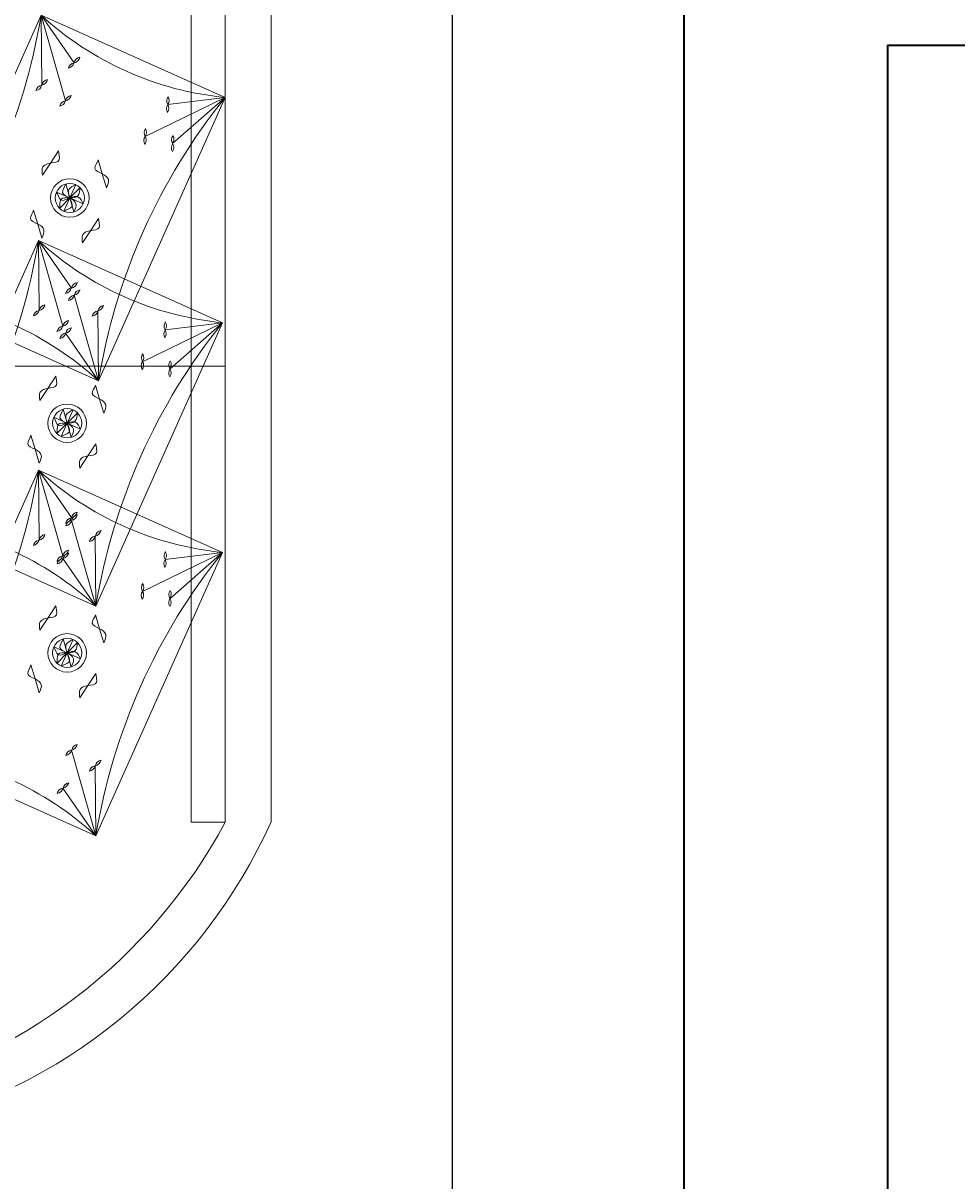
# Model space of a CAD drawing. Units: inches. Extents: x -61 to 1599, y -1316 to 257.
# Tile 82 of 204: x 240 to 268, y -407 to -373. Entities that reach past the tile are written whole.
import ezdxf

# ---------------------------------------------------------------- set-up
doc = ezdxf.new("R2010")
doc.units = ezdxf.units.IN
doc.header["$MEASUREMENT"] = 0
for name, color, linetype, lineweight in [('A-ANNO-DIMS', 2, 'Continuous', 18), ('FURNITURE', 83, 'Continuous', 18), ('WALLS', 4, 'Continuous', 35)]:
    doc.layers.add(name, color=color, linetype=linetype, lineweight=lineweight)
doc.styles.get("Standard").update_dxf_attribs({"font": 'arial.ttf'})
doc.dimstyles.get("Standard").update_dxf_attribs({"dimtxt": 0.18, "dimasz": 0.18, "dimexe": 0.18, "dimexo": 0.0625, "dimgap": 0.09, "dimtad": 0, "dimtih": 1, "dimtoh": 1, "dimdec": 0, "dimzin": 0, "dimdsep": 46, "dimlunit": 3, "dimtxsty": 'Standard', "dimcen": 0.09, "dimadec": 0, "dimazin": 0, "dimtfac": 1, "dimtdec": 0, "dimtofl": 0, "dimtmove": 0, "dimatfit": 3, "dimfxl": 1, "dimtolj": 1, "dimtzin": 0, "dimarcsym": 0})

# ---------------------------------------------------------------- blocks, each defined once
blk = doc.blocks.new('MASTER-BEDROOM-CONSOLE')
for p, q in [((0, 44.886), (23.587, 44.886)), ((23.587, 37.779), (23.587, 9.438)), ((23.587, 37.779), (24.943, 35.589)), ((24.943, 35.589), (24.943, 9.456)), ((18.162, 33.228), (18.879, 30.704)), ((18.162, 33.228), (19.133, 31.826)), ((18.162, 33.228), (18.181, 31.167)), ((23.587, 30.804), (21.228, 29.654)), ((23.587, 30.804), (21.894, 30.592)), ((23.587, 30.804), (22.038, 29.443)), ((18.441, 28.869), (18.678, 29.228)), ((18.203, 28.51), (18.441, 28.869)), ((19.963, 28.553), (19.841, 28.966)), ((20.085, 28.141), (19.963, 28.553)), ((19.008, 27.84), (18.615, 28.016)), ((19.008, 27.84), (18.886, 28.253)), ((19.184, 28.233), (19.008, 27.84)), ((19.309, 28.148), (19.008, 27.84)), ((19.008, 27.84), (18.707, 27.533)), ((19.008, 27.84), (18.833, 27.448)), ((19.401, 27.665), (19.008, 27.84)), ((19.13, 27.428), (19.008, 27.84)), ((18.061, 27.072), (17.939, 27.485)), ((18.183, 26.66), (18.061, 27.072)), ((19.618, 26.876), (19.855, 27.235)), ((19.38, 26.517), (19.618, 26.876)), ((18.084, 26.588), (18.801, 24.064)), ((18.084, 26.588), (19.055, 25.186)), ((18.084, 26.588), (18.103, 24.527)), ((14.429, 24.877), (15.978, 26.238)), ((14.429, 24.877), (16.788, 26.026)), ((14.429, 24.877), (16.122, 25.089)), ((19.854, 22.452), (19.137, 24.976)), ((19.854, 22.452), (19.835, 24.514)), ((23.509, 24.163), (21.15, 23.014)), ((23.509, 24.163), (21.816, 23.952)), ((23.509, 24.163), (21.96, 22.803)), ((19.854, 22.452), (18.883, 23.854)), ((0, 22.886), (23.587, 22.886)), ((18.362, 22.229), (18.6, 22.588)), ((18.125, 21.87), (18.362, 22.229)), ((19.885, 21.913), (19.763, 22.326)), ((20.007, 21.5), (19.885, 21.913)), ((18.93, 21.2), (18.808, 21.613)), ((19.105, 21.593), (18.93, 21.2)), ((19.23, 21.508), (18.93, 21.2)), ((18.93, 21.2), (18.537, 21.376)), ((18.93, 21.2), (18.629, 20.893)), ((18.93, 21.2), (18.754, 20.808)), ((19.322, 21.025), (18.93, 21.2)), ((19.052, 20.788), (18.93, 21.2)), ((17.983, 20.432), (17.861, 20.845)), ((19.54, 20.236), (19.777, 20.595)), ((18.105, 20.02), (17.983, 20.432)), ((19.302, 19.877), (19.54, 20.236)), ((18.084, 19.819), (18.801, 17.295)), ((18.084, 19.819), (19.055, 18.417)), ((18.084, 19.819), (18.103, 17.757)), ((14.351, 18.237), (15.9, 19.598)), ((14.351, 18.237), (16.71, 19.386)), ((14.351, 18.237), (16.043, 18.448)), ((19.776, 15.812), (19.059, 18.336)), ((19.776, 15.812), (19.757, 17.874)), ((19.776, 15.812), (18.804, 17.214)), ((23.509, 17.394), (21.15, 16.245)), ((23.509, 17.394), (21.816, 17.183)), ((23.509, 17.394), (21.96, 16.033)), ((18.362, 15.459), (18.6, 15.818)), ((18.125, 15.101), (18.362, 15.459)), ((19.885, 15.143), (19.763, 15.556)), ((20.007, 14.731), (19.885, 15.143)), ((18.93, 14.431), (18.808, 14.843)), ((19.105, 14.823), (18.93, 14.431)), ((19.23, 14.738), (18.93, 14.431)), ((18.93, 14.431), (18.537, 14.606)), ((18.93, 14.431), (18.629, 14.123)), ((18.93, 14.431), (18.754, 14.038)), ((19.322, 14.255), (18.93, 14.431)), ((19.052, 14.018), (18.93, 14.431)), ((17.983, 13.663), (17.861, 14.075)), ((18.105, 13.25), (17.983, 13.663)), ((19.54, 13.466), (19.777, 13.825)), ((19.302, 13.108), (19.54, 13.466)), ((14.351, 11.468), (15.9, 12.828)), ((14.351, 11.468), (16.71, 12.617)), ((14.351, 11.468), (16.043, 11.679)), ((19.776, 9.043), (19.059, 11.567)), ((19.776, 9.043), (19.757, 11.104)), ((19.776, 9.043), (18.804, 10.445)), ((22.587, 9.438), (23.587, 9.438)), ((1, 3.748), (0, 3.748))]:
    blk.add_line(p, q)
for points in [[(0, 3.748), (0, 62.524), (23.587, 62.524), (23.587, 9.438)], [(1, 3.748), (1, 61.524), (22.587, 61.524), (22.587, 9.438)]]:
    blk.add_lwpolyline(points)
for points in [[(14.429, 24.877), (18.162, 33.228), (23.587, 30.804), (19.854, 22.452)], [(14.351, 18.237), (18.084, 26.588), (23.509, 24.163), (19.776, 15.812)], [(14.351, 11.468), (18.084, 19.819), (23.509, 17.394), (19.776, 9.043)]]:
    blk.add_lwpolyline(points, close=True)
for centre, radius in [((19.008, 27.84), 0.567), ((19.008, 27.84), 0.567), ((19.008, 27.84), 0.43), ((18.93, 21.2), 0.567), ((18.93, 21.2), 0.567), ((18.93, 21.2), 0.43), ((18.93, 14.431), 0.567), ((18.93, 14.431), 0.567), ((18.93, 14.431), 0.43)]:
    blk.add_circle(centre, radius)
for centre, radius, start, end in [((0.46, 36.131), 17.938, 321.1446, 350.6879), ((24.495, 40.115), 9.356, 227.4013, 264.4312), ((19.167, 31.62), 0.209, 99.3213, 167.2974), ((18.925, 31.877), 0.214, 280.2125, 346.4062), ((19.095, 32.037), 0.214, 280.2125, 346.4062), ((19.338, 31.78), 0.209, 99.3213, 167.2974), ((18.215, 30.96), 0.209, 99.3213, 167.2974), ((17.973, 31.217), 0.214, 280.2125, 346.4062), ((18.143, 31.378), 0.214, 280.2125, 346.4062), ((18.385, 31.121), 0.209, 99.3213, 167.2974), ((18.841, 30.915), 0.214, 280.2125, 346.4062), ((19.083, 30.658), 0.209, 99.3213, 167.2974), ((37.556, 19.55), 17.938, 141.1446, 170.6879), ((22.077, 30.705), 0.214, 145.4264, 211.62), ((21.724, 30.714), 0.209, 324.5352, 32.5112), ((18.913, 30.498), 0.209, 99.3213, 167.2974), ((18.67, 30.755), 0.214, 280.2125, 346.4062), ((22.071, 30.471), 0.214, 145.4264, 211.62), ((21.718, 30.48), 0.209, 324.5352, 32.5112), ((21.411, 29.767), 0.214, 145.4264, 211.62), ((21.058, 29.776), 0.209, 324.5352, 32.5112), ((21.405, 29.533), 0.214, 145.4264, 211.62), ((21.052, 29.542), 0.209, 324.5352, 32.5112), ((22.215, 29.321), 0.214, 145.4264, 211.62), ((22.221, 29.555), 0.214, 145.4264, 211.62), ((21.861, 29.33), 0.209, 324.5352, 32.5112), ((21.867, 29.564), 0.209, 324.5352, 32.5112), ((0.382, 29.491), 17.938, 321.1446, 350.6879), ((16.155, 26.351), 0.209, 144.5352, 212.5112), ((15.802, 26.36), 0.214, 325.4264, 31.62), ((24.416, 33.475), 9.356, 227.4013, 264.4312), ((16.149, 26.117), 0.209, 144.5352, 212.5112), ((15.796, 26.126), 0.214, 325.4264, 31.62), ((16.959, 25.905), 0.209, 144.5352, 212.5112), ((16.965, 26.139), 0.209, 144.5352, 212.5112), ((16.605, 25.914), 0.214, 325.4264, 31.62), ((16.611, 26.148), 0.214, 325.4264, 31.62), ((16.298, 25.201), 0.209, 144.5352, 212.5112), ((15.945, 25.21), 0.214, 325.4264, 31.62), ((19.017, 25.397), 0.214, 280.2125, 346.4062), ((19.259, 25.14), 0.209, 99.3213, 167.2974), ((16.292, 24.967), 0.209, 144.5352, 212.5112), ((15.939, 24.976), 0.214, 325.4264, 31.62), ((19.089, 24.98), 0.209, 99.3213, 167.2974), ((18.847, 25.237), 0.214, 280.2125, 346.4062), ((19.175, 24.765), 0.214, 100.2125, 166.4062), ((18.933, 25.022), 0.209, 279.3213, 347.2974), ((19.103, 25.183), 0.209, 279.3213, 347.2974), ((19.346, 24.926), 0.214, 100.2125, 166.4062), ((13.521, 15.565), 9.356, 47.4013, 84.4312), ((18.065, 24.738), 0.214, 280.2125, 346.4062), ((18.307, 24.48), 0.209, 99.3213, 167.2974), ((19.801, 24.721), 0.209, 279.3213, 347.2974), ((20.043, 24.464), 0.214, 100.2125, 166.4062), ((18.137, 24.32), 0.209, 99.3213, 167.2974), ((17.894, 24.577), 0.214, 280.2125, 346.4062), ((19.873, 24.303), 0.214, 100.2125, 166.4062), ((19.631, 24.56), 0.209, 279.3213, 347.2974), ((18.834, 23.858), 0.209, 99.3213, 167.2974), ((18.592, 24.115), 0.214, 280.2125, 346.4062), ((18.763, 24.275), 0.214, 280.2125, 346.4062), ((19.005, 24.018), 0.209, 99.3213, 167.2974), ((18.849, 24.061), 0.209, 279.3213, 347.2974), ((19.091, 23.804), 0.214, 100.2125, 166.4062), ((37.478, 12.91), 17.938, 141.1446, 170.6879), ((21.993, 23.83), 0.214, 145.4264, 211.62), ((21.999, 24.065), 0.214, 145.4264, 211.62), ((21.64, 23.84), 0.209, 324.5352, 32.5112), ((21.646, 24.074), 0.209, 324.5352, 32.5112), ((18.921, 23.643), 0.214, 100.2125, 166.4062), ((18.678, 23.9), 0.209, 279.3213, 347.2974), ((21.332, 23.127), 0.214, 145.4264, 211.62), ((20.979, 23.136), 0.209, 324.5352, 32.5112), ((21.326, 22.892), 0.214, 145.4264, 211.62), ((20.973, 22.902), 0.209, 324.5352, 32.5112), ((22.142, 22.915), 0.214, 145.4264, 211.62), ((21.789, 22.924), 0.209, 324.5352, 32.5112), ((22.136, 22.681), 0.214, 145.4264, 211.62), ((21.783, 22.69), 0.209, 324.5352, 32.5112), ((0.382, 22.721), 17.938, 321.1446, 350.6879), ((16.076, 19.711), 0.209, 144.5352, 212.5112), ((15.723, 19.72), 0.214, 325.4264, 31.62), ((24.416, 26.706), 9.356, 227.4013, 264.4312), ((16.07, 19.476), 0.209, 144.5352, 212.5112), ((15.717, 19.486), 0.214, 325.4264, 31.62), ((16.886, 19.499), 0.209, 144.5352, 212.5112), ((16.533, 19.508), 0.214, 325.4264, 31.62), ((16.88, 19.265), 0.209, 144.5352, 212.5112), ((16.527, 19.274), 0.214, 325.4264, 31.62), ((16.214, 18.327), 0.209, 144.5352, 212.5112), ((16.22, 18.561), 0.209, 144.5352, 212.5112), ((15.861, 18.336), 0.214, 325.4264, 31.62), ((15.867, 18.57), 0.214, 325.4264, 31.62), ((19.017, 18.628), 0.214, 280.2125, 346.4062), ((19.259, 18.371), 0.209, 99.3213, 167.2974), ((19.025, 18.543), 0.209, 279.3213, 347.2974), ((19.267, 18.286), 0.214, 100.2125, 166.4062), ((13.443, 8.925), 9.356, 47.4013, 84.4312), ((19.089, 18.21), 0.209, 99.3213, 167.2974), ((18.847, 18.467), 0.214, 280.2125, 346.4062), ((19.097, 18.125), 0.214, 100.2125, 166.4062), ((18.855, 18.382), 0.209, 279.3213, 347.2974), ((18.137, 17.55), 0.209, 99.3213, 167.2974), ((17.894, 17.807), 0.214, 280.2125, 346.4062), ((18.065, 17.968), 0.214, 280.2125, 346.4062), ((18.307, 17.711), 0.209, 99.3213, 167.2974), ((19.795, 17.663), 0.214, 100.2125, 166.4062), ((19.552, 17.92), 0.209, 279.3213, 347.2974), ((19.723, 18.081), 0.209, 279.3213, 347.2974), ((19.965, 17.824), 0.214, 100.2125, 166.4062), ((18.763, 17.506), 0.214, 280.2125, 346.4062), ((19.005, 17.249), 0.209, 99.3213, 167.2974), ((21.999, 17.295), 0.214, 145.4264, 211.62), ((21.646, 17.304), 0.209, 324.5352, 32.5112), ((18.834, 17.088), 0.209, 99.3213, 167.2974), ((18.592, 17.345), 0.214, 280.2125, 346.4062), ((18.842, 17.003), 0.214, 100.2125, 166.4062), ((18.6, 17.26), 0.209, 279.3213, 347.2974), ((18.771, 17.421), 0.209, 279.3213, 347.2974), ((19.013, 17.164), 0.214, 100.2125, 166.4062), ((37.478, 6.14), 17.938, 141.1446, 170.6879), ((21.993, 17.061), 0.214, 145.4264, 211.62), ((21.64, 17.07), 0.209, 324.5352, 32.5112), ((21.332, 16.357), 0.214, 145.4264, 211.62), ((20.979, 16.366), 0.209, 324.5352, 32.5112), ((21.326, 16.123), 0.214, 145.4264, 211.62), ((20.973, 16.132), 0.209, 324.5352, 32.5112), ((22.142, 16.145), 0.214, 145.4264, 211.62), ((21.789, 16.155), 0.209, 324.5352, 32.5112), ((22.136, 15.911), 0.214, 145.4264, 211.62), ((21.783, 15.92), 0.209, 324.5352, 32.5112), ((16.076, 12.941), 0.209, 144.5352, 212.5112), ((15.723, 12.95), 0.214, 325.4264, 31.62), ((16.07, 12.707), 0.209, 144.5352, 212.5112), ((15.717, 12.716), 0.214, 325.4264, 31.62), ((16.886, 12.729), 0.209, 144.5352, 212.5112), ((16.533, 12.739), 0.214, 325.4264, 31.62), ((16.88, 12.495), 0.209, 144.5352, 212.5112), ((16.527, 12.504), 0.214, 325.4264, 31.62), ((16.214, 11.557), 0.209, 144.5352, 212.5112), ((16.22, 11.791), 0.209, 144.5352, 212.5112), ((15.861, 11.566), 0.214, 325.4264, 31.62), ((15.867, 11.801), 0.214, 325.4264, 31.62), ((19.025, 11.773), 0.209, 279.3213, 347.2974), ((19.267, 11.516), 0.214, 100.2125, 166.4062), ((13.443, 2.156), 9.356, 47.4013, 84.4312), ((19.097, 11.356), 0.214, 100.2125, 166.4062), ((18.855, 11.613), 0.209, 279.3213, 347.2974), ((19.723, 11.311), 0.209, 279.3213, 347.2974), ((19.965, 11.054), 0.214, 100.2125, 166.4062), ((19.795, 10.893), 0.214, 100.2125, 166.4062), ((19.552, 11.151), 0.209, 279.3213, 347.2974), ((18.771, 10.651), 0.209, 279.3213, 347.2974), ((19.013, 10.394), 0.214, 100.2125, 166.4062), ((18.842, 10.234), 0.214, 100.2125, 166.4062), ((18.6, 10.491), 0.209, 279.3213, 347.2974), ((10.308, 16.053), 16.053, 230.0449, 335.7344), ((9.449, 17.042), 16.053, 233.9382, 331.7264)]:
    blk.add_arc(centre, radius, start, end)
for points in [[(18.203, 28.51), (18.191, 28.604), (18.167, 28.791), (18.438, 28.884), (18.778, 28.897), (18.67, 29.157), (18.678, 29.228)], [(20.085, 28.141), (20.124, 28.226), (20.202, 28.398), (19.97, 28.566), (19.649, 28.679), (19.829, 28.896), (19.841, 28.966)], [(19.401, 27.665), (19.361, 27.75), (19.281, 27.921), (19.003, 27.854), (18.708, 27.683), (18.66, 27.961), (18.615, 28.016)], [(19.309, 28.148), (19.303, 28.054), (19.292, 27.866), (19.008, 27.825), (18.671, 27.876), (18.729, 27.6), (18.707, 27.533)], [(19.13, 27.428), (19.169, 27.514), (19.247, 27.685), (19.015, 27.854), (18.694, 27.966), (18.873, 28.183), (18.886, 28.253)], [(19.184, 28.233), (19.098, 28.193), (18.927, 28.113), (18.994, 27.835), (19.165, 27.54), (18.888, 27.492), (18.833, 27.448)], [(18.183, 26.66), (18.222, 26.746), (18.3, 26.917), (18.069, 27.086), (17.747, 27.198), (17.927, 27.415), (17.939, 27.485)], [(19.38, 26.517), (19.368, 26.611), (19.344, 26.798), (19.615, 26.891), (19.955, 26.904), (19.847, 27.164), (19.855, 27.235)], [(18.125, 21.87), (18.113, 21.964), (18.089, 22.151), (18.359, 22.244), (18.7, 22.257), (18.592, 22.517), (18.6, 22.588)], [(20.007, 21.5), (20.046, 21.586), (20.124, 21.758), (19.892, 21.926), (19.571, 22.039), (19.75, 22.256), (19.763, 22.326)], [(19.23, 21.508), (19.225, 21.414), (19.213, 21.226), (18.93, 21.185), (18.593, 21.236), (18.651, 20.96), (18.629, 20.893)], [(19.052, 20.788), (19.091, 20.874), (19.169, 21.045), (18.937, 21.214), (18.615, 21.326), (18.795, 21.543), (18.808, 21.613)], [(19.105, 21.593), (19.02, 21.553), (18.849, 21.473), (18.916, 21.195), (19.087, 20.9), (18.809, 20.852), (18.754, 20.808)], [(19.322, 21.025), (19.283, 21.11), (19.203, 21.281), (18.924, 21.214), (18.63, 21.043), (18.582, 21.321), (18.537, 21.376)], [(18.105, 20.02), (18.144, 20.105), (18.222, 20.277), (17.99, 20.445), (17.669, 20.558), (17.848, 20.775), (17.861, 20.845)], [(19.302, 19.877), (19.29, 19.971), (19.266, 20.158), (19.537, 20.251), (19.877, 20.264), (19.769, 20.524), (19.777, 20.595)], [(18.125, 15.101), (18.113, 15.194), (18.089, 15.381), (18.359, 15.474), (18.7, 15.488), (18.592, 15.748), (18.6, 15.818)], [(20.007, 14.731), (20.046, 14.817), (20.124, 14.988), (19.892, 15.157), (19.571, 15.269), (19.75, 15.486), (19.763, 15.556)], [(19.23, 14.738), (19.225, 14.644), (19.213, 14.456), (18.93, 14.416), (18.593, 14.466), (18.651, 14.191), (18.629, 14.123)], [(19.052, 14.018), (19.091, 14.104), (19.169, 14.276), (18.937, 14.444), (18.615, 14.557), (18.795, 14.773), (18.808, 14.843)], [(19.105, 14.823), (19.02, 14.784), (18.849, 14.704), (18.916, 14.425), (19.087, 14.131), (18.809, 14.083), (18.754, 14.038)], [(19.322, 14.255), (19.283, 14.341), (19.203, 14.511), (18.924, 14.445), (18.63, 14.274), (18.582, 14.551), (18.537, 14.606)], [(18.105, 13.25), (18.144, 13.336), (18.222, 13.508), (17.99, 13.676), (17.669, 13.788), (17.848, 14.005), (17.861, 14.075)], [(19.302, 13.108), (19.29, 13.201), (19.266, 13.388), (19.537, 13.481), (19.877, 13.495), (19.769, 13.755), (19.777, 13.825)]]:
    blk.add_open_spline(points, degree=3, knots=[0, 0, 0, 0, 0.249187, 0.498374, 0.766554, 1.034734, 1.034734, 1.034734, 1.034734])
blk = doc.blocks.new('*D687')
at = {"layer": 'A-ANNO-DIMS', "color": 0, "lineweight": -2, "transparency": 16777216}
for p, q in [((289.418, 181.677), (-61.077, 181.677)), ((-60.897, 181.497), (-60.897, -528.952)), ((-60.897, -1239.765), (-60.897, -529.316)), ((319.64, -1239.945), (-61.077, -1239.945))]:
    blk.add_line(p, q, dxfattribs=at)
at = {"layer": 'A-ANNO-DIMS', "color": 0, "transparency": 16777216}
for points in [[(-60.927, 181.497), (-60.867, 181.497), (-60.897, 181.677)], [(-60.927, -1239.765), (-60.867, -1239.765), (-60.897, -1239.945)]]:
    blk.add_solid(points, dxfattribs=at)
at = {"layer": 'DEFPOINTS', "color": 0, "transparency": 16777216}
for p in [(289.481, 181.677), (-60.897, -1239.945), (319.703, -1239.945)]:
    blk.add_point(p, dxfattribs=at)
at = {"layer": 'A-ANNO-DIMS', "color": 0, "transparency": 16777216, "insert": (-60.897, -529.134), "char_height": 0.18, "attachment_point": 5}
blk.add_mtext('\\A1;1421.6', dxfattribs=at)
blk = doc.blocks.new('*D699')
at = {"layer": 'A-ANNO-DIMS', "color": 0, "lineweight": -2, "transparency": 16777216}
for p, q in [((835.64, -167.169), (-61.077, -167.169)), ((-60.897, -167.349), (-60.897, -306.726)), ((-60.897, -446.466), (-60.897, -307.09)), ((841.64, -446.646), (-61.077, -446.646))]:
    blk.add_line(p, q, dxfattribs=at)
at = {"layer": 'A-ANNO-DIMS', "color": 0, "transparency": 16777216}
for points in [[(-60.927, -167.349), (-60.867, -167.349), (-60.897, -167.169)], [(-60.927, -446.466), (-60.867, -446.466), (-60.897, -446.646)]]:
    blk.add_solid(points, dxfattribs=at)
at = {"layer": 'DEFPOINTS', "color": 0, "transparency": 16777216}
for p in [(835.703, -167.169), (-60.897, -446.646), (841.703, -446.646)]:
    blk.add_point(p, dxfattribs=at)
at = {"layer": 'A-ANNO-DIMS', "color": 0, "transparency": 16777216, "insert": (-60.897, -306.908), "char_height": 0.18, "attachment_point": 5}
blk.add_mtext('\\A1;279.5', dxfattribs=at)
blk = doc.blocks.new('*D701')
at = {"layer": 'A-ANNO-DIMS', "color": 0, "lineweight": -2, "transparency": 16777216}
for p, q in [((215.752, -616.882), (215.752, 257.457)), ((252.882, -616.882), (252.882, 257.457)), ((215.932, 257.277), (233.924, 257.277)), ((252.702, 257.277), (234.711, 257.277))]:
    blk.add_line(p, q, dxfattribs=at)
at = {"layer": 'A-ANNO-DIMS', "color": 0, "transparency": 16777216}
for points in [[(215.932, 257.307), (215.932, 257.247), (215.752, 257.277)], [(252.702, 257.307), (252.702, 257.247), (252.882, 257.277)]]:
    blk.add_solid(points, dxfattribs=at)
at = {"layer": 'DEFPOINTS', "color": 0, "transparency": 16777216}
for p in [(252.882, 257.277), (215.752, -616.945), (252.882, -616.945)]:
    blk.add_point(p, dxfattribs=at)
at = {"layer": 'A-ANNO-DIMS', "color": 0, "transparency": 16777216, "insert": (234.317, 257.277), "char_height": 0.18, "attachment_point": 5}
blk.add_mtext('\\A1;37.13', dxfattribs=at)

msp = doc.modelspace()

# ---------------------------------------------------------------- linework, layer by layer
at = {"layer": 'WALLS'}
for p, q in [((259.7028, -288.3229), (259.7028, -432.3229)), ((265.7028, -373.3229), (319.7028, -373.3229)), ((265.7028, -373.3229), (265.7028, -432.3229))]:
    msp.add_line(p, q, dxfattribs=at)

# ---------------------------------------------------------------- block references
at = {"layer": 'FURNITURE'}
msp.add_blockref('MASTER-BEDROOM-CONSOLE', (222.602, -405.667), dxfattribs=at)

# ---------------------------------------------------------------- dimensions: what is measured, and where the dimension line sits
at = {"layer": 'A-ANNO-DIMS'}
dim = msp.add_linear_dim(base=(252.8825, 257.2771), p1=(215.7521, -616.9446), p2=(252.8825, -616.9446), dimstyle='Standard', override={"dimdec": 2, "dimlfac": 1, "dimrnd": 0, "dimzin": 0, "dimdsep": 46, "dimlunit": 2}, dxfattribs=at)
dim.commit()
dim.dimension.update_dxf_attribs({"geometry": '*D701', "text_midpoint": (234.3173, 257.2771)})
for base, p1, p2, picture, middle in [((-60.8972, -1239.9446), (289.4807, 181.6771), (319.7028, -1239.9446), '*D687', (-60.8972, -529.1337)), ((-60.8972, -446.6462), (835.7028, -167.169), (841.7028, -446.6462), '*D699', (-60.8972, -306.9076))]:
    dim = msp.add_linear_dim(base=base, p1=p1, p2=p2, angle=90, dimstyle='Standard', override={"dimdec": 1, "dimlfac": 1, "dimrnd": 0, "dimzin": 0, "dimdsep": 46, "dimlunit": 2}, dxfattribs=at)
    dim.commit()
    dim.dimension.update_dxf_attribs({"geometry": picture, "text_midpoint": middle})

doc.saveas('drawing.dxf')
